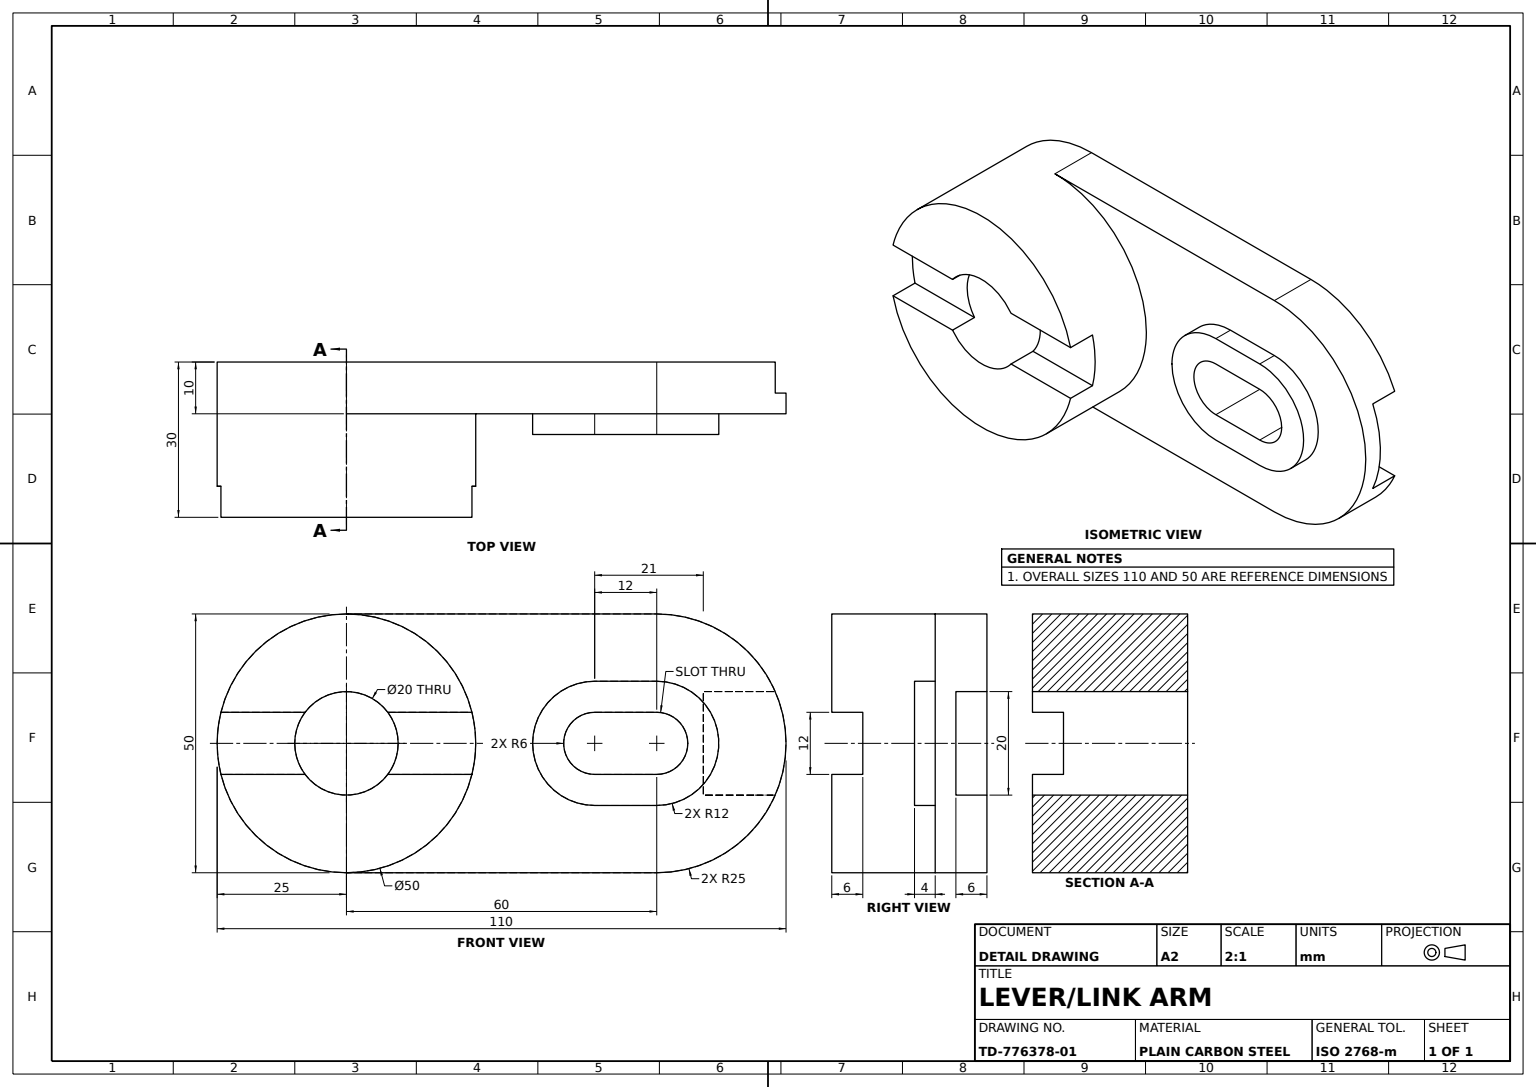
from build123d import *

# Parameters (mm, degrees)
ARM_PLATE_DEPTH      = 10
HUB_FRONT_SKETCH_R   = 25
HUB_BOSS_FRONT_DEPTH = 10
HUB_START            = 20
HUB_BACK_SKETCH_R    = 25
HUB_BOSS_BACK_DEPTH  = 20
HUB_CROSS_SLOT_DEPTH = 6
BORE_SKETCH_R        = 10
BORE_20_DEPTH        = 30
SLOT_BOSS_DEPTH      = 4
ARM_SLOT_12MM_DEPTH  = 20
END_NOTCH_DEPTH      = 94.541434669
END_NOTCH_DEPTH_BACK = 6


with BuildPart() as part:
    # Arm Profile Sketch → Arm Plate (new body)
    with BuildSketch(Plane.XY):
        with BuildLine():
            Line((60, 25), (0, 25))
            Line((0, 25), (0, -25))
            Line((0, -25), (60, -25))
            ThreePointArc((60, -25), (85, 0), (60, 25))
        make_face()
    extrude(amount=ARM_PLATE_DEPTH)

    # Hub Front Sketch → Hub Boss Front (add)
    with BuildSketch(Plane.XY.offset(10)):
        Circle(HUB_FRONT_SKETCH_R)
    extrude(amount=-HUB_BOSS_FRONT_DEPTH)

    # Hub Back Sketch → Hub Boss Back (add)
    with BuildSketch(Plane.XY.offset(10).offset(HUB_START)):
        Circle(HUB_BACK_SKETCH_R)
    extrude(amount=-HUB_BOSS_BACK_DEPTH)

    # Hub Cross Slot Sketch → Hub Cross Slot (cut)
    with BuildSketch(Plane.XY.offset(30)):
        with BuildLine():
            ThreePointArc((24.269322199, -6), (24.816658266, -3.022163548), (25, 0))
            ThreePointArc((25, 0), (24.816658266, 3.022163548), (24.269322199, 6))
            Line((24.269322199, 6), (8, 6))
            ThreePointArc((8, 6), (0, 10), (-8, 6))
            Line((-8, 6), (-24.269322199, 6))
            ThreePointArc((-24.269322199, 6), (-24.816658266, 3.022163548), (-25, 0))
            ThreePointArc((-25, 0), (-24.816658266, -3.022163548), (-24.269322199, -6))
            Line((-24.269322199, -6), (-8, -6))
            ThreePointArc((-8, -6), (0, -10), (8, -6))
            Line((8, -6), (24.269322199, -6))
        make_face()
    extrude(amount=-HUB_CROSS_SLOT_DEPTH, mode=Mode.SUBTRACT)

    # Bore Sketch → Bore Ø20 (cut)
    with BuildSketch(Plane.XY.offset(24)):
        Circle(BORE_SKETCH_R)
    extrude(amount=-BORE_20_DEPTH, mode=Mode.SUBTRACT)

    # Slot Boss Sketch → Slot Boss (add)
    with BuildSketch(Plane.XY.offset(10)):
        with BuildLine():
            Line((48, 12), (60, 12))
            ThreePointArc((60, 12), (72, 0), (60, -12))
            Line((60, -12), (48, -12))
            ThreePointArc((48, -12), (36, 0), (48, 12))
        make_face()
    extrude(amount=SLOT_BOSS_DEPTH)

    # Arm Slot Sketch → Arm Slot 12mm (cut)
    with BuildSketch(Plane.XY.offset(14)):
        with BuildLine():
            Line((48, 6), (60, 6))
            ThreePointArc((60, 6), (66, 0), (60, -6))
            Line((60, -6), (48, -6))
            ThreePointArc((48, -6), (42, 0), (48, 6))
        make_face()
    extrude(amount=-ARM_SLOT_12MM_DEPTH, mode=Mode.SUBTRACT)

    # End Notch Sketch → End Notch (cut, two sides: drawn at the far end of the back side and taken through both)
    with BuildSketch(Plane(origin=(0, 0, 0), x_dir=(-1, 0, 0), z_dir=(0, 0, -1)).offset(-END_NOTCH_DEPTH_BACK)):
        Polygon((-319.806592277, -10), (-82.912878475, -10), (-79, -10), (-69, -10), (-69, 10), (-79, 10), (-82.912878475, 10), (-319.806592277, 10), (-793.594019881, 10), (-793.594019881, -10), align=None)
    extrude(amount=END_NOTCH_DEPTH + END_NOTCH_DEPTH_BACK, mode=Mode.SUBTRACT)


solid = part.part
